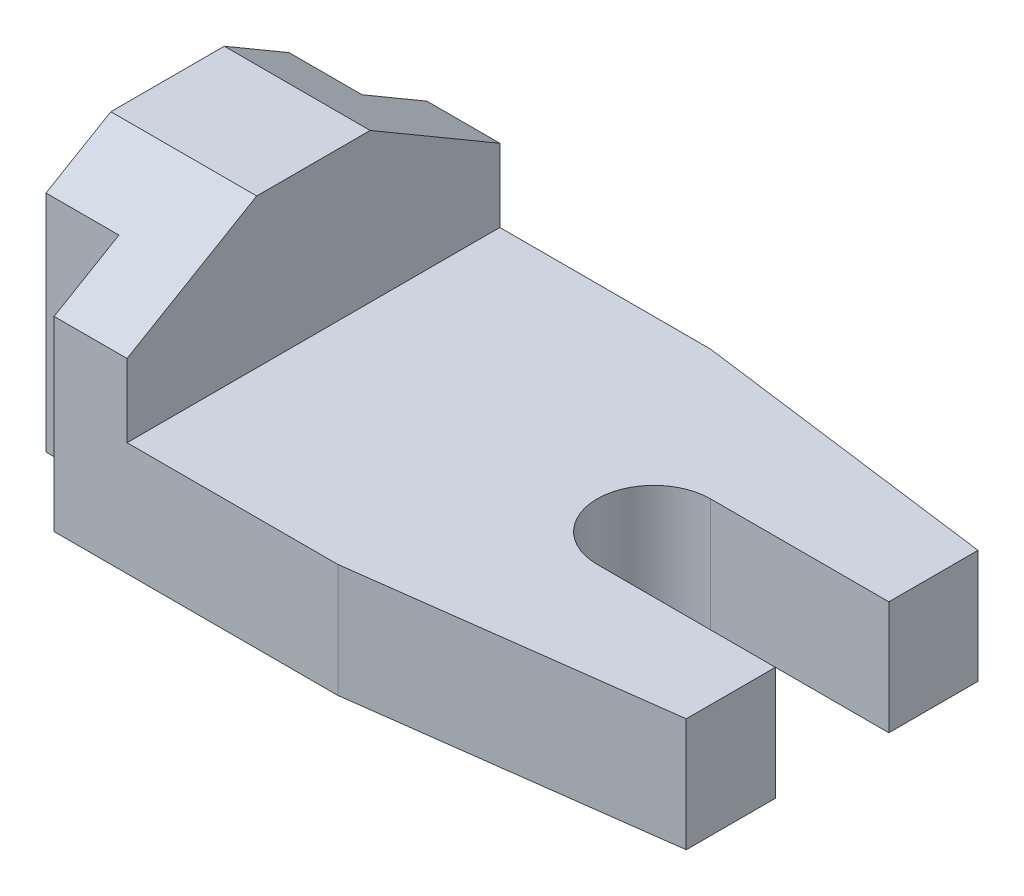
ISO-10303-21;
HEADER;
FILE_DESCRIPTION(('STEP AP214'),'2;1');
FILE_NAME('part.step','',(''),(''),'','','');
FILE_SCHEMA(('AUTOMOTIVE_DESIGN { 1 0 10303 214 1 1 1 1 }'));
ENDSEC;
DATA;
#1=APPLICATION_CONTEXT('core data for automotive mechanical design processes');
#2=APPLICATION_PROTOCOL_DEFINITION('international standard','automotive_design',2000,#1);
#3=PRODUCT_CONTEXT('',#1,'mechanical');
#4=PRODUCT('Part','Part','',(#3));
#5=PRODUCT_RELATED_PRODUCT_CATEGORY('part','',(#4));
#6=PRODUCT_DEFINITION_FORMATION('','',#4);
#7=PRODUCT_DEFINITION_CONTEXT('part definition',#1,'design');
#8=PRODUCT_DEFINITION('design','',#6,#7);
#9=PRODUCT_DEFINITION_SHAPE('','',#8);
#10=(LENGTH_UNIT() NAMED_UNIT(*) SI_UNIT(.MILLI.,.METRE.));
#11=(NAMED_UNIT(*) PLANE_ANGLE_UNIT() SI_UNIT($,.RADIAN.));
#12=(NAMED_UNIT(*) SI_UNIT($,.STERADIAN.) SOLID_ANGLE_UNIT());
#13=UNCERTAINTY_MEASURE_WITH_UNIT(LENGTH_MEASURE(1.E-05),#10,'distance_accuracy_value','');
#14=(GEOMETRIC_REPRESENTATION_CONTEXT(3) GLOBAL_UNCERTAINTY_ASSIGNED_CONTEXT((#13)) GLOBAL_UNIT_ASSIGNED_CONTEXT((#10,
#11,#12)) REPRESENTATION_CONTEXT('',''));
#15=CARTESIAN_POINT('',(0.,0.,0.));
#16=DIRECTION('',(0.,0.,1.));
#17=DIRECTION('',(1.,0.,0.));
#18=AXIS2_PLACEMENT_3D('',#15,#16,#17);
#19=CARTESIAN_POINT('',(-45.5274134647977,14.,0.));
#20=DIRECTION('',(1.,0.,0.));
#21=DIRECTION('',(0.,0.,-1.));
#22=AXIS2_PLACEMENT_3D('',#19,#20,#21);
#23=PLANE('',#22);
#24=DIRECTION('',(0.,-0.505294515224669,0.862946958325867));
#25=VECTOR('',#24,1.);
#26=CARTESIAN_POINT('',(-45.5274134647977,32.3687244222741,-2.47332622537585));
#27=LINE('',#26,#25);
#28=CARTESIAN_POINT('',(-45.5274134647978,27.6843622111371,5.52667377462414));
#29=VERTEX_POINT('',#28);
#30=CARTESIAN_POINT('',(-45.5274134647977,23.,13.5266737746241));
#31=VERTEX_POINT('',#30);
#32=EDGE_CURVE('E203',#29,#31,#27,.T.);
#33=ORIENTED_EDGE('',*,*,#32,.F.);
#34=DIRECTION('',(0.,-1.,0.));
#35=VECTOR('',#34,1.);
#36=CARTESIAN_POINT('',(-45.5274134647977,14.,5.52667377462414));
#37=LINE('',#36,#35);
#38=CARTESIAN_POINT('',(-45.5274134647977,0.,5.52667377462414));
#39=VERTEX_POINT('',#38);
#40=EDGE_CURVE('E179',#29,#39,#37,.T.);
#41=ORIENTED_EDGE('',*,*,#40,.T.);
#42=DIRECTION('',(0.,0.,1.));
#43=VECTOR('',#42,1.);
#44=CARTESIAN_POINT('',(-45.5274134647977,0.,0.));
#45=LINE('',#44,#43);
#46=CARTESIAN_POINT('',(-45.5274134647977,0.,13.5266737746241));
#47=VERTEX_POINT('',#46);
#48=EDGE_CURVE('E235',#39,#47,#45,.T.);
#49=ORIENTED_EDGE('',*,*,#48,.T.);
#50=DIRECTION('',(0.,-1.,0.));
#51=VECTOR('',#50,1.);
#52=CARTESIAN_POINT('',(-45.5274134647977,14.,13.5266737746241));
#53=LINE('',#52,#51);
#54=EDGE_CURVE('E11',#31,#47,#53,.T.);
#55=ORIENTED_EDGE('',*,*,#54,.F.);
#56=EDGE_LOOP('',(#33,#41,#49,#55));
#57=FACE_BOUND('',#56,.T.);
#58=ADVANCED_FACE('F43',(#57),#23,.F.);
#59=DIRECTION('',(0.,-1.,0.));
#60=VECTOR('',#59,1.);
#61=CARTESIAN_POINT('',(-45.5274134647977,14.,-24.4733262253759));
#62=LINE('',#61,#60);
#63=CARTESIAN_POINT('',(-45.5274134647977,27.6843622111371,-24.4733262253758));
#64=VERTEX_POINT('',#63);
#65=CARTESIAN_POINT('',(-45.5274134647977,0.,-24.4733262253759));
#66=VERTEX_POINT('',#65);
#67=EDGE_CURVE('E293',#64,#66,#62,.T.);
#68=ORIENTED_EDGE('',*,*,#67,.F.);
#69=DIRECTION('',(0.,0.505294515224669,0.862946958325868));
#70=VECTOR('',#69,1.);
#71=CARTESIAN_POINT('',(-45.5274134647977,32.3687244222741,-16.4733262253758));
#72=LINE('',#71,#70);
#73=CARTESIAN_POINT('',(-45.5274134647977,23.,-32.4733262253759));
#74=VERTEX_POINT('',#73);
#75=EDGE_CURVE('E204',#74,#64,#72,.T.);
#76=ORIENTED_EDGE('',*,*,#75,.F.);
#77=DIRECTION('',(0.,-1.,0.));
#78=VECTOR('',#77,1.);
#79=CARTESIAN_POINT('',(-45.5274134647977,14.,-32.4733262253759));
#80=LINE('',#79,#78);
#81=CARTESIAN_POINT('',(-45.5274134647977,0.,-32.4733262253759));
#82=VERTEX_POINT('',#81);
#83=EDGE_CURVE('E295',#74,#82,#80,.T.);
#84=ORIENTED_EDGE('',*,*,#83,.T.);
#85=DIRECTION('',(0.,0.,1.));
#86=VECTOR('',#85,1.);
#87=CARTESIAN_POINT('',(-45.5274134647977,0.,0.));
#88=LINE('',#87,#86);
#89=EDGE_CURVE('E283',#82,#66,#88,.T.);
#90=ORIENTED_EDGE('',*,*,#89,.T.);
#91=EDGE_LOOP('',(#68,#76,#84,#90));
#92=FACE_BOUND('',#91,.T.);
#93=ADVANCED_FACE('F370',(#92),#23,.F.);
#94=CARTESIAN_POINT('',(0.,14.,0.));
#95=DIRECTION('',(0.,1.,0.));
#96=DIRECTION('',(0.,0.,1.));
#97=AXIS2_PLACEMENT_3D('',#94,#95,#96);
#98=PLANE('',#97);
#99=DIRECTION('',(-1.,0.,0.));
#100=VECTOR('',#99,1.);
#101=CARTESIAN_POINT('',(0.,14.,-32.4733262253759));
#102=LINE('',#101,#100);
#103=CARTESIAN_POINT('',(-10.5274134647977,14.,-32.4733262253759));
#104=VERTEX_POINT('',#103);
#105=CARTESIAN_POINT('',(-36.5274134647977,14.,-32.4733262253759));
#106=VERTEX_POINT('',#105);
#107=EDGE_CURVE('E59',#104,#106,#102,.T.);
#108=ORIENTED_EDGE('',*,*,#107,.T.);
#109=DIRECTION('',(0.,0.,1.));
#110=VECTOR('',#109,1.);
#111=CARTESIAN_POINT('',(-36.5274134647977,14.,0.));
#112=LINE('',#111,#110);
#113=CARTESIAN_POINT('',(-36.5274134647977,14.,13.5266737746241));
#114=VERTEX_POINT('',#113);
#115=EDGE_CURVE('E65',#106,#114,#112,.T.);
#116=ORIENTED_EDGE('',*,*,#115,.T.);
#117=DIRECTION('',(1.,0.,0.));
#118=VECTOR('',#117,1.);
#119=CARTESIAN_POINT('',(0.,14.,13.5266737746241));
#120=LINE('',#119,#118);
#121=CARTESIAN_POINT('',(-10.5274134647977,14.,13.5266737746241));
#122=VERTEX_POINT('',#121);
#123=EDGE_CURVE('E231',#114,#122,#120,.T.);
#124=ORIENTED_EDGE('',*,*,#123,.T.);
#125=DIRECTION('',(0.991454295542544,0.,-0.130454512571388));
#126=VECTOR('',#125,1.);
#127=CARTESIAN_POINT('',(1.57037622910732,14.,11.9348593412156));
#128=LINE('',#127,#126);
#129=CARTESIAN_POINT('',(27.4725865352023,14.,8.52667377462413));
#130=VERTEX_POINT('',#129);
#131=EDGE_CURVE('E232',#122,#130,#128,.T.);
#132=ORIENTED_EDGE('',*,*,#131,.T.);
#133=DIRECTION('',(0.,0.,1.));
#134=VECTOR('',#133,1.);
#135=CARTESIAN_POINT('',(27.4725865352023,14.,0.));
#136=LINE('',#135,#134);
#137=CARTESIAN_POINT('',(27.4725865352023,14.,-2.47332622537586));
#138=VERTEX_POINT('',#137);
#139=EDGE_CURVE('E238',#138,#130,#136,.T.);
#140=ORIENTED_EDGE('',*,*,#139,.F.);
#141=DIRECTION('',(1.,0.,0.));
#142=VECTOR('',#141,1.);
#143=CARTESIAN_POINT('',(0.,14.,-2.47332622537587));
#144=LINE('',#143,#142);
#145=CARTESIAN_POINT('',(5.47258653520229,14.,-2.47332622537587));
#146=VERTEX_POINT('',#145);
#147=EDGE_CURVE('E241',#146,#138,#144,.T.);
#148=ORIENTED_EDGE('',*,*,#147,.F.);
#149=CARTESIAN_POINT('',(5.47258653520229,14.,-9.47332622537587));
#150=DIRECTION('',(0.,1.,0.));
#151=DIRECTION('',(0.,0.,1.));
#152=AXIS2_PLACEMENT_3D('',#149,#150,#151);
#153=CIRCLE('',#152,7.);
#154=CARTESIAN_POINT('',(5.47258653520229,14.,-16.4733262253759));
#155=VERTEX_POINT('',#154);
#156=EDGE_CURVE('E242',#155,#146,#153,.T.);
#157=ORIENTED_EDGE('',*,*,#156,.F.);
#158=DIRECTION('',(1.,0.,0.));
#159=VECTOR('',#158,1.);
#160=CARTESIAN_POINT('',(0.,14.,-16.4733262253759));
#161=LINE('',#160,#159);
#162=CARTESIAN_POINT('',(27.4725865352023,14.,-16.4733262253759));
#163=VERTEX_POINT('',#162);
#164=EDGE_CURVE('E250',#155,#163,#161,.T.);
#165=ORIENTED_EDGE('',*,*,#164,.T.);
#166=DIRECTION('',(0.,0.,1.));
#167=VECTOR('',#166,1.);
#168=CARTESIAN_POINT('',(27.4725865352023,14.,0.));
#169=LINE('',#168,#167);
#170=CARTESIAN_POINT('',(27.4725865352023,14.,-27.4733262253759));
#171=VERTEX_POINT('',#170);
#172=EDGE_CURVE('E248',#171,#163,#169,.T.);
#173=ORIENTED_EDGE('',*,*,#172,.F.);
#174=DIRECTION('',(0.991454295542544,0.,0.130454512571387));
#175=VECTOR('',#174,1.);
#176=CARTESIAN_POINT('',(4.02093032416709,14.,-30.55907046367));
#177=LINE('',#176,#175);
#178=EDGE_CURVE('E255',#104,#171,#177,.T.);
#179=ORIENTED_EDGE('',*,*,#178,.F.);
#180=EDGE_LOOP('',(#108,#116,#124,#132,#140,#148,#157,#165,#173,#179));
#181=FACE_BOUND('',#180,.T.);
#182=ADVANCED_FACE('F328',(#181),#98,.T.);
#183=CARTESIAN_POINT('',(0.,14.,13.5266737746241));
#184=DIRECTION('',(0.,0.,-1.));
#185=DIRECTION('',(-1.,0.,0.));
#186=AXIS2_PLACEMENT_3D('',#183,#184,#185);
#187=PLANE('',#186);
#188=DIRECTION('',(1.,0.,0.));
#189=VECTOR('',#188,1.);
#190=CARTESIAN_POINT('',(0.,0.,13.5266737746241));
#191=LINE('',#190,#189);
#192=CARTESIAN_POINT('',(-10.5274134647977,0.,13.5266737746241));
#193=VERTEX_POINT('',#192);
#194=EDGE_CURVE('E259',#47,#193,#191,.T.);
#195=ORIENTED_EDGE('',*,*,#194,.T.);
#196=DIRECTION('',(0.,-1.,0.));
#197=VECTOR('',#196,1.);
#198=CARTESIAN_POINT('',(-10.5274134647977,14.,13.5266737746241));
#199=LINE('',#198,#197);
#200=EDGE_CURVE('E51',#122,#193,#199,.T.);
#201=ORIENTED_EDGE('',*,*,#200,.F.);
#202=ORIENTED_EDGE('',*,*,#123,.F.);
#203=DIRECTION('',(0.,-1.,0.));
#204=VECTOR('',#203,1.);
#205=CARTESIAN_POINT('',(-36.5274134647977,23.,13.5266737746241));
#206=LINE('',#205,#204);
#207=CARTESIAN_POINT('',(-36.5274134647977,23.,13.5266737746241));
#208=VERTEX_POINT('',#207);
#209=EDGE_CURVE('E226',#208,#114,#206,.T.);
#210=ORIENTED_EDGE('',*,*,#209,.F.);
#211=DIRECTION('',(1.,0.,0.));
#212=VECTOR('',#211,1.);
#213=CARTESIAN_POINT('',(-36.5274134647977,23.,13.5266737746241));
#214=LINE('',#213,#212);
#215=EDGE_CURVE('E218',#31,#208,#214,.T.);
#216=ORIENTED_EDGE('',*,*,#215,.F.);
#217=ORIENTED_EDGE('',*,*,#54,.T.);
#218=EDGE_LOOP('',(#195,#201,#202,#210,#216,#217));
#219=FACE_BOUND('',#218,.T.);
#220=ADVANCED_FACE('F44',(#219),#187,.F.);
#221=CARTESIAN_POINT('',(1.57037622910732,14.,11.9348593412156));
#222=DIRECTION('',(-0.130454512571388,0.,-0.991454295542544));
#223=DIRECTION('',(-0.991454295542544,0.,0.130454512571388));
#224=AXIS2_PLACEMENT_3D('',#221,#222,#223);
#225=PLANE('',#224);
#226=DIRECTION('',(0.991454295542544,0.,-0.130454512571388));
#227=VECTOR('',#226,1.);
#228=CARTESIAN_POINT('',(1.57037622910732,0.,11.9348593412156));
#229=LINE('',#228,#227);
#230=CARTESIAN_POINT('',(27.4725865352023,0.,8.52667377462413));
#231=VERTEX_POINT('',#230);
#232=EDGE_CURVE('E258',#193,#231,#229,.T.);
#233=ORIENTED_EDGE('',*,*,#232,.T.);
#234=DIRECTION('',(0.,-1.,0.));
#235=VECTOR('',#234,1.);
#236=CARTESIAN_POINT('',(27.4725865352023,14.,8.52667377462413));
#237=LINE('',#236,#235);
#238=EDGE_CURVE('E307',#130,#231,#237,.T.);
#239=ORIENTED_EDGE('',*,*,#238,.F.);
#240=ORIENTED_EDGE('',*,*,#131,.F.);
#241=ORIENTED_EDGE('',*,*,#200,.T.);
#242=EDGE_LOOP('',(#233,#239,#240,#241));
#243=FACE_BOUND('',#242,.T.);
#244=ADVANCED_FACE('F314',(#243),#225,.F.);
#245=CARTESIAN_POINT('',(27.4725865352023,14.,0.));
#246=DIRECTION('',(1.,0.,0.));
#247=DIRECTION('',(0.,0.,-1.));
#248=AXIS2_PLACEMENT_3D('',#245,#246,#247);
#249=PLANE('',#248);
#250=DIRECTION('',(0.,0.,1.));
#251=VECTOR('',#250,1.);
#252=CARTESIAN_POINT('',(27.4725865352023,0.,0.));
#253=LINE('',#252,#251);
#254=CARTESIAN_POINT('',(27.4725865352023,0.,-2.47332622537586));
#255=VERTEX_POINT('',#254);
#256=EDGE_CURVE('E263',#255,#231,#253,.T.);
#257=ORIENTED_EDGE('',*,*,#256,.F.);
#258=DIRECTION('',(0.,-1.,0.));
#259=VECTOR('',#258,1.);
#260=CARTESIAN_POINT('',(27.4725865352023,14.,-2.47332622537586));
#261=LINE('',#260,#259);
#262=EDGE_CURVE('E310',#138,#255,#261,.T.);
#263=ORIENTED_EDGE('',*,*,#262,.F.);
#264=ORIENTED_EDGE('',*,*,#139,.T.);
#265=ORIENTED_EDGE('',*,*,#238,.T.);
#266=EDGE_LOOP('',(#257,#263,#264,#265));
#267=FACE_BOUND('',#266,.T.);
#268=ADVANCED_FACE('F323',(#267),#249,.T.);
#269=CARTESIAN_POINT('',(0.,14.,-2.47332622537587));
#270=DIRECTION('',(0.,0.,-1.));
#271=DIRECTION('',(-1.,0.,0.));
#272=AXIS2_PLACEMENT_3D('',#269,#270,#271);
#273=PLANE('',#272);
#274=DIRECTION('',(1.,0.,0.));
#275=VECTOR('',#274,1.);
#276=CARTESIAN_POINT('',(0.,0.,-2.47332622537587));
#277=LINE('',#276,#275);
#278=CARTESIAN_POINT('',(5.47258653520229,0.,-2.47332622537587));
#279=VERTEX_POINT('',#278);
#280=EDGE_CURVE('E266',#279,#255,#277,.T.);
#281=ORIENTED_EDGE('',*,*,#280,.F.);
#282=DIRECTION('',(0.,-1.,0.));
#283=VECTOR('',#282,1.);
#284=CARTESIAN_POINT('',(5.47258653520229,14.,-2.47332622537587));
#285=LINE('',#284,#283);
#286=EDGE_CURVE('E304',#146,#279,#285,.T.);
#287=ORIENTED_EDGE('',*,*,#286,.F.);
#288=ORIENTED_EDGE('',*,*,#147,.T.);
#289=ORIENTED_EDGE('',*,*,#262,.T.);
#290=EDGE_LOOP('',(#281,#287,#288,#289));
#291=FACE_BOUND('',#290,.T.);
#292=ADVANCED_FACE('F331',(#291),#273,.T.);
#293=CARTESIAN_POINT('',(5.47258653520229,14.,-9.47332622537587));
#294=DIRECTION('',(0.,-1.,0.));
#295=DIRECTION('',(0.,0.,-1.));
#296=AXIS2_PLACEMENT_3D('',#293,#294,#295);
#297=CYLINDRICAL_SURFACE('',#296,7.);
#298=CARTESIAN_POINT('',(5.47258653520229,0.,-9.47332622537587));
#299=DIRECTION('',(0.,1.,0.));
#300=DIRECTION('',(0.,0.,1.));
#301=AXIS2_PLACEMENT_3D('',#298,#299,#300);
#302=CIRCLE('',#301,7.);
#303=CARTESIAN_POINT('',(5.47258653520229,0.,-16.4733262253759));
#304=VERTEX_POINT('',#303);
#305=EDGE_CURVE('E267',#304,#279,#302,.T.);
#306=ORIENTED_EDGE('',*,*,#305,.F.);
#307=DIRECTION('',(0.,-1.,0.));
#308=VECTOR('',#307,1.);
#309=CARTESIAN_POINT('',(5.47258653520229,14.,-16.4733262253759));
#310=LINE('',#309,#308);
#311=EDGE_CURVE('E303',#155,#304,#310,.T.);
#312=ORIENTED_EDGE('',*,*,#311,.F.);
#313=ORIENTED_EDGE('',*,*,#156,.T.);
#314=ORIENTED_EDGE('',*,*,#286,.T.);
#315=EDGE_LOOP('',(#306,#312,#313,#314));
#316=FACE_BOUND('',#315,.T.);
#317=ADVANCED_FACE('F332',(#316),#297,.F.);
#318=CARTESIAN_POINT('',(0.,14.,-16.4733262253759));
#319=DIRECTION('',(0.,0.,-1.));
#320=DIRECTION('',(-1.,0.,0.));
#321=AXIS2_PLACEMENT_3D('',#318,#319,#320);
#322=PLANE('',#321);
#323=DIRECTION('',(1.,0.,0.));
#324=VECTOR('',#323,1.);
#325=CARTESIAN_POINT('',(0.,0.,-16.4733262253759));
#326=LINE('',#325,#324);
#327=CARTESIAN_POINT('',(27.4725865352023,0.,-16.4733262253759));
#328=VERTEX_POINT('',#327);
#329=EDGE_CURVE('E275',#304,#328,#326,.T.);
#330=ORIENTED_EDGE('',*,*,#329,.T.);
#331=DIRECTION('',(0.,-1.,0.));
#332=VECTOR('',#331,1.);
#333=CARTESIAN_POINT('',(27.4725865352023,14.,-16.4733262253759));
#334=LINE('',#333,#332);
#335=EDGE_CURVE('E301',#163,#328,#334,.T.);
#336=ORIENTED_EDGE('',*,*,#335,.F.);
#337=ORIENTED_EDGE('',*,*,#164,.F.);
#338=ORIENTED_EDGE('',*,*,#311,.T.);
#339=EDGE_LOOP('',(#330,#336,#337,#338));
#340=FACE_BOUND('',#339,.T.);
#341=ADVANCED_FACE('F339',(#340),#322,.F.);
#342=CARTESIAN_POINT('',(27.4725865352023,14.,0.));
#343=DIRECTION('',(1.,0.,0.));
#344=DIRECTION('',(0.,0.,-1.));
#345=AXIS2_PLACEMENT_3D('',#342,#343,#344);
#346=PLANE('',#345);
#347=DIRECTION('',(0.,0.,1.));
#348=VECTOR('',#347,1.);
#349=CARTESIAN_POINT('',(27.4725865352023,0.,0.));
#350=LINE('',#349,#348);
#351=CARTESIAN_POINT('',(27.4725865352023,0.,-27.4733262253759));
#352=VERTEX_POINT('',#351);
#353=EDGE_CURVE('E273',#352,#328,#350,.T.);
#354=ORIENTED_EDGE('',*,*,#353,.F.);
#355=DIRECTION('',(0.,-1.,0.));
#356=VECTOR('',#355,1.);
#357=CARTESIAN_POINT('',(27.4725865352023,14.,-27.4733262253759));
#358=LINE('',#357,#356);
#359=EDGE_CURVE('E299',#171,#352,#358,.T.);
#360=ORIENTED_EDGE('',*,*,#359,.F.);
#361=ORIENTED_EDGE('',*,*,#172,.T.);
#362=ORIENTED_EDGE('',*,*,#335,.T.);
#363=EDGE_LOOP('',(#354,#360,#361,#362));
#364=FACE_BOUND('',#363,.T.);
#365=ADVANCED_FACE('F344',(#364),#346,.T.);
#366=CARTESIAN_POINT('',(4.02093032416709,14.,-30.55907046367));
#367=DIRECTION('',(0.130454512571387,0.,-0.991454295542544));
#368=DIRECTION('',(-0.991454295542544,0.,-0.130454512571387));
#369=AXIS2_PLACEMENT_3D('',#366,#367,#368);
#370=PLANE('',#369);
#371=DIRECTION('',(0.991454295542544,0.,0.130454512571387));
#372=VECTOR('',#371,1.);
#373=CARTESIAN_POINT('',(4.02093032416709,0.,-30.55907046367));
#374=LINE('',#373,#372);
#375=CARTESIAN_POINT('',(-10.5274134647977,0.,-32.4733262253759));
#376=VERTEX_POINT('',#375);
#377=EDGE_CURVE('E279',#376,#352,#374,.T.);
#378=ORIENTED_EDGE('',*,*,#377,.F.);
#379=DIRECTION('',(0.,-1.,0.));
#380=VECTOR('',#379,1.);
#381=CARTESIAN_POINT('',(-10.5274134647977,14.,-32.4733262253759));
#382=LINE('',#381,#380);
#383=EDGE_CURVE('E300',#104,#376,#382,.T.);
#384=ORIENTED_EDGE('',*,*,#383,.F.);
#385=ORIENTED_EDGE('',*,*,#178,.T.);
#386=ORIENTED_EDGE('',*,*,#359,.T.);
#387=EDGE_LOOP('',(#378,#384,#385,#386));
#388=FACE_BOUND('',#387,.T.);
#389=ADVANCED_FACE('F346',(#388),#370,.T.);
#390=CARTESIAN_POINT('',(0.,14.,-32.4733262253759));
#391=DIRECTION('',(0.,0.,1.));
#392=DIRECTION('',(1.,0.,0.));
#393=AXIS2_PLACEMENT_3D('',#390,#391,#392);
#394=PLANE('',#393);
#395=ORIENTED_EDGE('',*,*,#83,.F.);
#396=DIRECTION('',(-1.,0.,0.));
#397=VECTOR('',#396,1.);
#398=CARTESIAN_POINT('',(-45.5274134647977,23.,-32.4733262253759));
#399=LINE('',#398,#397);
#400=CARTESIAN_POINT('',(-36.5274134647977,23.,-32.4733262253759));
#401=VERTEX_POINT('',#400);
#402=EDGE_CURVE('E225',#401,#74,#399,.T.);
#403=ORIENTED_EDGE('',*,*,#402,.F.);
#404=DIRECTION('',(0.,-1.,0.));
#405=VECTOR('',#404,1.);
#406=CARTESIAN_POINT('',(-36.5274134647977,23.,-32.4733262253759));
#407=LINE('',#406,#405);
#408=EDGE_CURVE('E224',#401,#106,#407,.T.);
#409=ORIENTED_EDGE('',*,*,#408,.T.);
#410=ORIENTED_EDGE('',*,*,#107,.F.);
#411=ORIENTED_EDGE('',*,*,#383,.T.);
#412=DIRECTION('',(-1.,0.,0.));
#413=VECTOR('',#412,1.);
#414=CARTESIAN_POINT('',(0.,0.,-32.4733262253759));
#415=LINE('',#414,#413);
#416=EDGE_CURVE('E281',#376,#82,#415,.T.);
#417=ORIENTED_EDGE('',*,*,#416,.T.);
#418=EDGE_LOOP('',(#395,#403,#409,#410,#411,#417));
#419=FACE_BOUND('',#418,.T.);
#420=ADVANCED_FACE('F347',(#419),#394,.F.);
#421=CARTESIAN_POINT('',(0.,14.,-24.4733262253759));
#422=DIRECTION('',(0.,0.,1.));
#423=DIRECTION('',(1.,0.,0.));
#424=AXIS2_PLACEMENT_3D('',#421,#422,#423);
#425=PLANE('',#424);
#426=DIRECTION('',(-1.,0.,0.));
#427=VECTOR('',#426,1.);
#428=CARTESIAN_POINT('',(0.,0.,-24.4733262253759));
#429=LINE('',#428,#427);
#430=CARTESIAN_POINT('',(-54.5274134647977,0.,-24.4733262253759));
#431=VERTEX_POINT('',#430);
#432=EDGE_CURVE('E284',#66,#431,#429,.T.);
#433=ORIENTED_EDGE('',*,*,#432,.T.);
#434=DIRECTION('',(0.,-1.,0.));
#435=VECTOR('',#434,1.);
#436=CARTESIAN_POINT('',(-54.5274134647977,14.,-24.4733262253759));
#437=LINE('',#436,#435);
#438=CARTESIAN_POINT('',(-54.5274134647977,27.6843622111371,-24.4733262253759));
#439=VERTEX_POINT('',#438);
#440=EDGE_CURVE('E177',#439,#431,#437,.T.);
#441=ORIENTED_EDGE('',*,*,#440,.F.);
#442=DIRECTION('',(1.,0.,0.));
#443=VECTOR('',#442,1.);
#444=CARTESIAN_POINT('',(-54.5274134647977,27.6843622111371,-24.4733262253759));
#445=LINE('',#444,#443);
#446=EDGE_CURVE('E186',#439,#64,#445,.T.);
#447=ORIENTED_EDGE('',*,*,#446,.T.);
#448=ORIENTED_EDGE('',*,*,#67,.T.);
#449=EDGE_LOOP('',(#433,#441,#447,#448));
#450=FACE_BOUND('',#449,.T.);
#451=ADVANCED_FACE('F359',(#450),#425,.F.);
#452=CARTESIAN_POINT('',(-54.5274134647977,14.,0.));
#453=DIRECTION('',(1.,0.,0.));
#454=DIRECTION('',(0.,0.,-1.));
#455=AXIS2_PLACEMENT_3D('',#452,#453,#454);
#456=PLANE('',#455);
#457=DIRECTION('',(0.,0.,1.));
#458=VECTOR('',#457,1.);
#459=CARTESIAN_POINT('',(-54.5274134647977,0.,0.));
#460=LINE('',#459,#458);
#461=CARTESIAN_POINT('',(-54.5274134647977,0.,5.52667377462414));
#462=VERTEX_POINT('',#461);
#463=EDGE_CURVE('E176',#431,#462,#460,.T.);
#464=ORIENTED_EDGE('',*,*,#463,.T.);
#465=DIRECTION('',(0.,-1.,0.));
#466=VECTOR('',#465,1.);
#467=CARTESIAN_POINT('',(-54.5274134647977,14.,5.52667377462414));
#468=LINE('',#467,#466);
#469=CARTESIAN_POINT('',(-54.5274134647977,27.6843622111371,5.52667377462414));
#470=VERTEX_POINT('',#469);
#471=EDGE_CURVE('E170',#470,#462,#468,.T.);
#472=ORIENTED_EDGE('',*,*,#471,.F.);
#473=DIRECTION('',(0.,0.505294515224669,-0.862946958325867));
#474=VECTOR('',#473,1.);
#475=CARTESIAN_POINT('',(-54.5274134647977,32.3687244222741,-2.47332622537586));
#476=LINE('',#475,#474);
#477=CARTESIAN_POINT('',(-54.5274134647977,32.3687244222741,-2.47332622537586));
#478=VERTEX_POINT('',#477);
#479=EDGE_CURVE('E175',#470,#478,#476,.T.);
#480=ORIENTED_EDGE('',*,*,#479,.T.);
#481=DIRECTION('',(0.,0.,-1.));
#482=VECTOR('',#481,1.);
#483=CARTESIAN_POINT('',(-54.5274134647977,32.3687244222741,-16.4733262253759));
#484=LINE('',#483,#482);
#485=CARTESIAN_POINT('',(-54.5274134647977,32.3687244222741,-16.4733262253759));
#486=VERTEX_POINT('',#485);
#487=EDGE_CURVE('E191',#478,#486,#484,.T.);
#488=ORIENTED_EDGE('',*,*,#487,.T.);
#489=DIRECTION('',(0.,-0.505294515224669,-0.862946958325867));
#490=VECTOR('',#489,1.);
#491=CARTESIAN_POINT('',(-54.5274134647977,27.6843622111371,-24.4733262253759));
#492=LINE('',#491,#490);
#493=EDGE_CURVE('E196',#486,#439,#492,.T.);
#494=ORIENTED_EDGE('',*,*,#493,.T.);
#495=ORIENTED_EDGE('',*,*,#440,.T.);
#496=EDGE_LOOP('',(#464,#472,#480,#488,#494,#495));
#497=FACE_BOUND('',#496,.T.);
#498=ADVANCED_FACE('F169',(#497),#456,.F.);
#499=CARTESIAN_POINT('',(0.,14.,5.52667377462414));
#500=DIRECTION('',(0.,0.,-1.));
#501=DIRECTION('',(-1.,0.,0.));
#502=AXIS2_PLACEMENT_3D('',#499,#500,#501);
#503=PLANE('',#502);
#504=DIRECTION('',(1.,0.,0.));
#505=VECTOR('',#504,1.);
#506=CARTESIAN_POINT('',(0.,0.,5.52667377462414));
#507=LINE('',#506,#505);
#508=EDGE_CURVE('E236',#462,#39,#507,.T.);
#509=ORIENTED_EDGE('',*,*,#508,.T.);
#510=ORIENTED_EDGE('',*,*,#40,.F.);
#511=DIRECTION('',(1.,0.,0.));
#512=VECTOR('',#511,1.);
#513=CARTESIAN_POINT('',(-54.5274134647977,27.6843622111371,5.52667377462414));
#514=LINE('',#513,#512);
#515=EDGE_CURVE('E182',#470,#29,#514,.T.);
#516=ORIENTED_EDGE('',*,*,#515,.F.);
#517=ORIENTED_EDGE('',*,*,#471,.T.);
#518=EDGE_LOOP('',(#509,#510,#516,#517));
#519=FACE_BOUND('',#518,.T.);
#520=ADVANCED_FACE('F183',(#519),#503,.F.);
#521=CARTESIAN_POINT('',(0.,0.,0.));
#522=DIRECTION('',(0.,1.,0.));
#523=DIRECTION('',(0.,0.,1.));
#524=AXIS2_PLACEMENT_3D('',#521,#522,#523);
#525=PLANE('',#524);
#526=ORIENTED_EDGE('',*,*,#89,.F.);
#527=ORIENTED_EDGE('',*,*,#416,.F.);
#528=ORIENTED_EDGE('',*,*,#377,.T.);
#529=ORIENTED_EDGE('',*,*,#353,.T.);
#530=ORIENTED_EDGE('',*,*,#329,.F.);
#531=ORIENTED_EDGE('',*,*,#305,.T.);
#532=ORIENTED_EDGE('',*,*,#280,.T.);
#533=ORIENTED_EDGE('',*,*,#256,.T.);
#534=ORIENTED_EDGE('',*,*,#232,.F.);
#535=ORIENTED_EDGE('',*,*,#194,.F.);
#536=ORIENTED_EDGE('',*,*,#48,.F.);
#537=ORIENTED_EDGE('',*,*,#508,.F.);
#538=ORIENTED_EDGE('',*,*,#463,.F.);
#539=ORIENTED_EDGE('',*,*,#432,.F.);
#540=EDGE_LOOP('',(#526,#527,#528,#529,#530,#531,#532,#533,#534,#535,#536,#537,#538,#539));
#541=FACE_BOUND('',#540,.T.);
#542=ADVANCED_FACE('F318',(#541),#525,.F.);
#543=CARTESIAN_POINT('',(-36.5274134647977,23.,-32.4733262253759));
#544=DIRECTION('',(-1.,0.,0.));
#545=DIRECTION('',(0.,0.,1.));
#546=AXIS2_PLACEMENT_3D('',#543,#544,#545);
#547=PLANE('',#546);
#548=ORIENTED_EDGE('',*,*,#115,.F.);
#549=ORIENTED_EDGE('',*,*,#408,.F.);
#550=DIRECTION('',(0.,0.505294515224669,0.862946958325868));
#551=VECTOR('',#550,1.);
#552=CARTESIAN_POINT('',(-36.5274134647977,32.3687244222741,-16.4733262253758));
#553=LINE('',#552,#551);
#554=CARTESIAN_POINT('',(-36.5274134647977,32.3687244222741,-16.4733262253758));
#555=VERTEX_POINT('',#554);
#556=EDGE_CURVE('E215',#401,#555,#553,.T.);
#557=ORIENTED_EDGE('',*,*,#556,.T.);
#558=DIRECTION('',(0.,0.,1.));
#559=VECTOR('',#558,1.);
#560=CARTESIAN_POINT('',(-36.5274134647977,32.3687244222741,-16.4733262253758));
#561=LINE('',#560,#559);
#562=CARTESIAN_POINT('',(-36.5274134647977,32.3687244222741,-2.47332622537586));
#563=VERTEX_POINT('',#562);
#564=EDGE_CURVE('E207',#555,#563,#561,.T.);
#565=ORIENTED_EDGE('',*,*,#564,.T.);
#566=DIRECTION('',(0.,-0.505294515224669,0.862946958325867));
#567=VECTOR('',#566,1.);
#568=CARTESIAN_POINT('',(-36.5274134647977,32.3687244222741,-2.47332622537586));
#569=LINE('',#568,#567);
#570=EDGE_CURVE('E189',#563,#208,#569,.T.);
#571=ORIENTED_EDGE('',*,*,#570,.T.);
#572=ORIENTED_EDGE('',*,*,#209,.T.);
#573=EDGE_LOOP('',(#548,#549,#557,#565,#571,#572));
#574=FACE_BOUND('',#573,.T.);
#575=ADVANCED_FACE('F353',(#574),#547,.F.);
#576=CARTESIAN_POINT('',(-45.5274134647977,32.3687244222741,-2.47332622537585));
#577=DIRECTION('',(0.,0.862946958325867,0.505294515224669));
#578=DIRECTION('',(0.,-0.505294515224669,0.862946958325867));
#579=AXIS2_PLACEMENT_3D('',#576,#577,#578);
#580=PLANE('',#579);
#581=ORIENTED_EDGE('',*,*,#570,.F.);
#582=DIRECTION('',(1.,0.,0.));
#583=VECTOR('',#582,1.);
#584=CARTESIAN_POINT('',(-45.5274134647977,32.3687244222741,-2.47332622537585));
#585=LINE('',#584,#583);
#586=EDGE_CURVE('E194',#478,#563,#585,.T.);
#587=ORIENTED_EDGE('',*,*,#586,.F.);
#588=ORIENTED_EDGE('',*,*,#479,.F.);
#589=ORIENTED_EDGE('',*,*,#515,.T.);
#590=ORIENTED_EDGE('',*,*,#32,.T.);
#591=ORIENTED_EDGE('',*,*,#215,.T.);
#592=EDGE_LOOP('',(#581,#587,#588,#589,#590,#591));
#593=FACE_BOUND('',#592,.T.);
#594=ADVANCED_FACE('F195',(#593),#580,.T.);
#595=CARTESIAN_POINT('',(-45.5274134647977,32.3687244222741,-16.4733262253758));
#596=DIRECTION('',(0.,1.,0.));
#597=DIRECTION('',(0.,0.,1.));
#598=AXIS2_PLACEMENT_3D('',#595,#596,#597);
#599=PLANE('',#598);
#600=ORIENTED_EDGE('',*,*,#564,.F.);
#601=DIRECTION('',(1.,0.,0.));
#602=VECTOR('',#601,1.);
#603=CARTESIAN_POINT('',(-45.5274134647977,32.3687244222741,-16.4733262253758));
#604=LINE('',#603,#602);
#605=EDGE_CURVE('E209',#486,#555,#604,.T.);
#606=ORIENTED_EDGE('',*,*,#605,.F.);
#607=ORIENTED_EDGE('',*,*,#487,.F.);
#608=ORIENTED_EDGE('',*,*,#586,.T.);
#609=EDGE_LOOP('',(#600,#606,#607,#608));
#610=FACE_BOUND('',#609,.T.);
#611=ADVANCED_FACE('F438',(#610),#599,.T.);
#612=CARTESIAN_POINT('',(-45.5274134647977,32.3687244222741,-16.4733262253758));
#613=DIRECTION('',(0.,0.862946958325867,-0.505294515224669));
#614=DIRECTION('',(0.,0.505294515224669,0.862946958325868));
#615=AXIS2_PLACEMENT_3D('',#612,#613,#614);
#616=PLANE('',#615);
#617=ORIENTED_EDGE('',*,*,#556,.F.);
#618=ORIENTED_EDGE('',*,*,#402,.T.);
#619=ORIENTED_EDGE('',*,*,#75,.T.);
#620=ORIENTED_EDGE('',*,*,#446,.F.);
#621=ORIENTED_EDGE('',*,*,#493,.F.);
#622=ORIENTED_EDGE('',*,*,#605,.T.);
#623=EDGE_LOOP('',(#617,#618,#619,#620,#621,#622));
#624=FACE_BOUND('',#623,.T.);
#625=ADVANCED_FACE('F364',(#624),#616,.T.);
#626=CLOSED_SHELL('',(#58,#93,#182,#220,#244,#268,#292,#317,#341,#365,#389,#420,#451,#498,#520,
#542,#575,#594,#611,#625));
#627=MANIFOLD_SOLID_BREP('B2',#626);
#628=ADVANCED_BREP_SHAPE_REPRESENTATION('',(#18,#627),#14);
#629=SHAPE_DEFINITION_REPRESENTATION(#9,#628);
ENDSEC;
END-ISO-10303-21;
